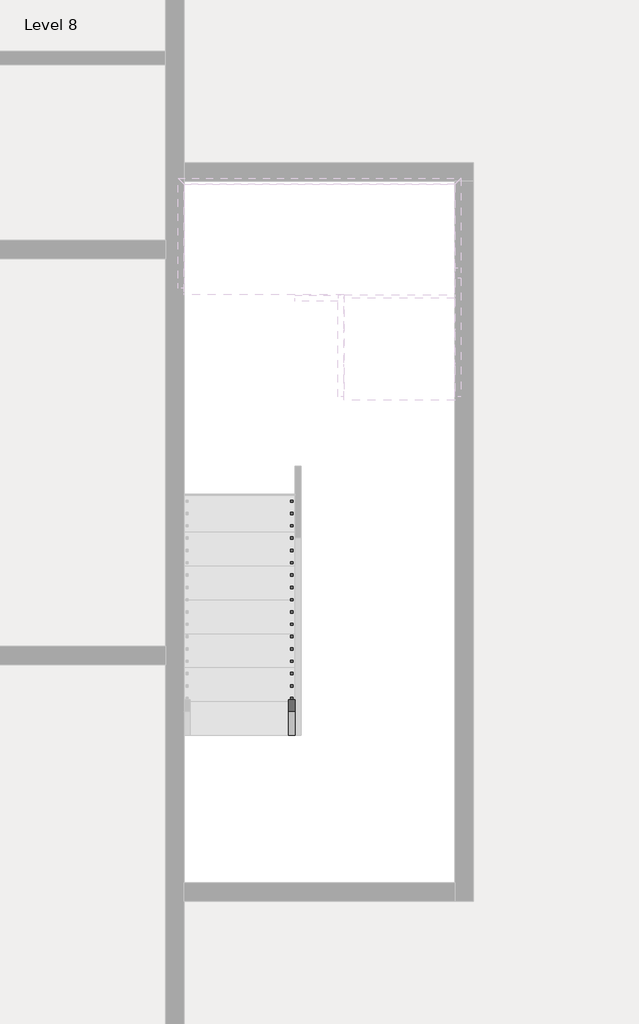
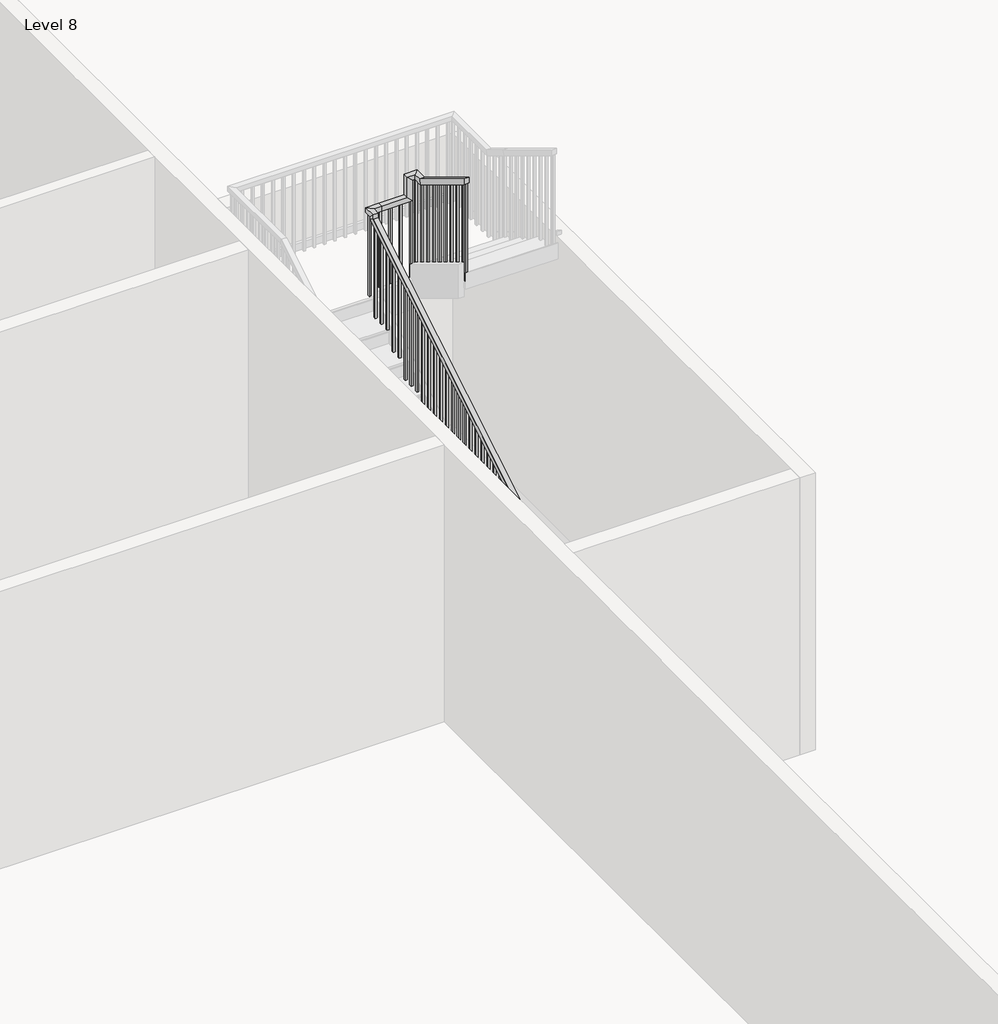
# One storey, part 5 of 8: 1 railing.
"""IFC4 building model written with IfcOpenShell, lengths in millimetres."""

from ifc_helpers import new_model, si_unit, frame, origin, place, context, project, spatial, polyline, outline, extrude, faceted_brep, element, save

model = new_model("IFC4")

# Units and contexts
model_context = context("Model", 3, world=origin())
ifc_project = project(units=[si_unit("LENGTHUNIT", "METRE", prefix="MILLI")], contexts=[model_context])

# Site, building, storey
site = spatial("IfcSite", under=ifc_project)
building = spatial("IfcBuilding", under=site)
storey = spatial("IfcBuildingStorey", under=building, Name="Level 8", Elevation=46570.6172466)

# Railing
placement = place(None, origin())
element("IfcRailing", 1, ObjectType="Handrail - Rectangular", at=placement, inside=storey, context=model_context, shape_type="SolidModel", body=[
    faceted_brep([(-2753.8415084, -23154.3851539, 47654.3505799), (-2753.8415084, -23154.3851539, 47594.9491197), (-2703.0415084, -23154.3851539, 47594.9491197), (-2703.0415084, -23154.3851539, 47654.3505799), (-2753.8415084, -19598.3851539, 49809.5020951), (-2753.8415084, -19547.5851539, 49780.8885136), (-2703.0415084, -19547.5851539, 49780.8885136), (-2703.0415084, -19598.3851539, 49809.5020951), (-2753.8415084, -19598.3851539, 49855.6839133), (-2753.8415084, -19547.5851539, 49804.8839133), (-2703.0415084, -19547.5851539, 49804.8839133), (-2703.0415084, -19598.3851539, 49855.6839133), (-2753.8415084, -19471.3851539, 49855.6839133), (-2753.8415084, -19471.3851539, 49804.8839133), (-2703.0415084, -19522.1851539, 49804.8839133), (-2703.0415084, -19522.1851539, 49855.6839133), (-2626.8415084, -19471.3851539, 49855.6839133), (-2626.8415084, -19471.3851539, 49804.8839133), (-2626.8415084, -19522.1851539, 49804.8839133), (-2626.8415084, -19522.1851539, 49855.6839133), (-2372.8415084, -19471.3851539, 49855.6839133), (-2322.0415084, -19471.3851539, 49804.8839133), (-2322.0415084, -19522.1851539, 49804.8839133), (-2372.8415084, -19522.1851539, 49855.6839133), (-2372.8415084, -19471.3851539, 50071.1990648), (-2322.0415084, -19471.3851539, 50020.3990648), (-2322.0415084, -19522.1851539, 50020.3990648), (-2372.8415084, -19522.1851539, 50071.1990648), (-2245.8415084, -19471.3851539, 50071.1990648), (-2245.8415084, -19471.3851539, 50020.3990648), (-2296.6415084, -19522.1851539, 50020.3990648), (-2296.6415084, -19522.1851539, 50071.1990648), (-2245.8415084, -19598.3851539, 50071.1990648), (-2245.8415084, -19612.5775633, 50020.3990648), (-2296.6415084, -19612.5775633, 50020.3990648), (-2296.6415084, -19598.3851539, 50071.1990648), (-2245.8415084, -20360.3851539, 50533.0172466), (-2296.6415084, -20360.3851539, 50533.0172466), (-2296.6415084, -20360.3851539, 50473.6157863), (-2245.8415084, -20360.3851539, 50473.6157863)], [[[0, 1, 2, 3]], [[1, 0, 4, 5]], [[2, 1, 5, 6]], [[3, 2, 6, 7]], [[0, 3, 7, 4]], [[5, 4, 8, 9]], [[6, 5, 9, 10]], [[7, 6, 10, 11]], [[4, 7, 11, 8]], [[9, 8, 12, 13]], [[10, 9, 13, 14]], [[11, 10, 14, 15]], [[8, 11, 15, 12]], [[13, 12, 16, 17]], [[14, 13, 17, 18]], [[15, 14, 18, 19]], [[12, 15, 19, 16]], [[17, 16, 20, 21]], [[18, 17, 21, 22]], [[19, 18, 22, 23]], [[16, 19, 23, 20]], [[21, 20, 24, 25]], [[22, 21, 25, 26]], [[23, 22, 26, 27]], [[20, 23, 27, 24]], [[25, 24, 28, 29]], [[26, 25, 29, 30]], [[27, 26, 30, 31]], [[24, 27, 31, 28]], [[29, 28, 32, 33]], [[30, 29, 33, 34]], [[31, 30, 34, 35]], [[28, 31, 35, 32]], [[36, 37, 38, 39]], [[33, 32, 36, 39]], [[34, 33, 39, 38]], [[35, 34, 38, 37]], [[32, 35, 37, 36]]]),
    extrude(outline(polyline([(-20319.1101539, 50448.6006348), (-20300.0601539, 50437.0551803), (-20300.0601539, 49449.2839133), (-20319.1101539, 49449.2839133), (-20319.1101539, 50448.6006348)])), frame((-2280.7665084, 0.0, 0.0), z_axis=(1.0, 0.0, 0.0), x_axis=(0.0, 1.0, 0.0)), (0.0, 0.0, 1.0), 19.05),
    extrude(outline(polyline([(-20217.5101539, 50387.0248773), (-20198.4601539, 50375.4794227), (-20198.4601539, 49449.2839133), (-20217.5101539, 49449.2839133), (-20217.5101539, 50387.0248773)])), frame((-2280.7665084, 0.0, 0.0), z_axis=(1.0, 0.0, 0.0), x_axis=(0.0, 1.0, 0.0)), (0.0, 0.0, 1.0), 19.05),
    extrude(outline(polyline([(-20115.9101539, 50325.4491197), (-20096.8601539, 50313.9036651), (-20096.8601539, 49449.2839133), (-20115.9101539, 49449.2839133), (-20115.9101539, 50325.4491197)])), frame((-2280.7665084, 0.0, 0.0), z_axis=(1.0, 0.0, 0.0), x_axis=(0.0, 1.0, 0.0)), (0.0, 0.0, 1.0), 19.05),
    extrude(outline(polyline([(-20014.3101539, 50263.8733621), (-19995.2601539, 50252.3279076), (-19995.2601539, 49279.9505799), (-20014.3101539, 49279.9505799), (-20014.3101539, 50263.8733621)])), frame((-2280.7665084, 0.0, 0.0), z_axis=(1.0, 0.0, 0.0), x_axis=(0.0, 1.0, 0.0)), (0.0, 0.0, 1.0), 19.05),
    extrude(outline(polyline([(-19912.7101539, 50202.2976045), (-19893.6601539, 50190.75215), (-19893.6601539, 49279.9505799), (-19912.7101539, 49279.9505799), (-19912.7101539, 50202.2976045)])), frame((-2280.7665084, 0.0, 0.0), z_axis=(1.0, 0.0, 0.0), x_axis=(0.0, 1.0, 0.0)), (0.0, 0.0, 1.0), 19.05),
    extrude(outline(polyline([(-19811.1101539, 50140.721847), (-19792.0601539, 50129.1763924), (-19792.0601539, 49279.9505799), (-19811.1101539, 49279.9505799), (-19811.1101539, 50140.721847)])), frame((-2280.7665084, 0.0, 0.0), z_axis=(1.0, 0.0, 0.0), x_axis=(0.0, 1.0, 0.0)), (0.0, 0.0, 1.0), 19.05),
    extrude(outline(polyline([(-19709.5101539, 50079.1460894), (-19690.4601539, 50067.6006348), (-19690.4601539, 49110.6172466), (-19709.5101539, 49110.6172466), (-19709.5101539, 50079.1460894)])), frame((-2280.7665084, 0.0, 0.0), z_axis=(1.0, 0.0, 0.0), x_axis=(0.0, 1.0, 0.0)), (0.0, 0.0, 1.0), 19.05),
    extrude(outline(polyline([(-19607.9101539, 50017.5703318), (-19588.8601539, 50006.0248773), (-19588.8601539, 49110.6172466), (-19607.9101539, 49110.6172466), (-19607.9101539, 50017.5703318)])), frame((-2280.7665084, 0.0, 0.0), z_axis=(1.0, 0.0, 0.0), x_axis=(0.0, 1.0, 0.0)), (0.0, 0.0, 1.0), 19.05),
    extrude(outline(polyline([(-2331.5665084, -19506.3101539), (-2331.5665084, -19487.2601539), (-2312.5165084, -19487.2601539), (-2312.5165084, -19506.3101539), (-2331.5665084, -19506.3101539)])), frame((0.0, 0.0, 48941.2839133), z_axis=(0.0, 0.0, 1.0), x_axis=(1.0, 0.0, 0.0)), (0.0, 0.0, 1.0), 1079.1151515),
    extrude(outline(polyline([(-2433.1665084, -19506.3101539), (-2433.1665084, -19487.2601539), (-2414.1165084, -19487.2601539), (-2414.1165084, -19506.3101539), (-2433.1665084, -19506.3101539)])), frame((0.0, 0.0, 48941.2839133), z_axis=(0.0, 0.0, 1.0), x_axis=(1.0, 0.0, 0.0)), (0.0, 0.0, 1.0), 863.6),
    extrude(outline(polyline([(-2534.7665084, -19506.3101539), (-2534.7665084, -19487.2601539), (-2515.7165084, -19487.2601539), (-2515.7165084, -19506.3101539), (-2534.7665084, -19506.3101539)])), frame((0.0, 0.0, 48941.2839133), z_axis=(0.0, 0.0, 1.0), x_axis=(1.0, 0.0, 0.0)), (0.0, 0.0, 1.0), 863.6),
    extrude(outline(polyline([(-2636.3665084, -19506.3101539), (-2636.3665084, -19487.2601539), (-2617.3165084, -19487.2601539), (-2617.3165084, -19506.3101539), (-2636.3665084, -19506.3101539)])), frame((0.0, 0.0, 48941.2839133), z_axis=(0.0, 0.0, 1.0), x_axis=(1.0, 0.0, 0.0)), (0.0, 0.0, 1.0), 863.6),
    extrude(outline(polyline([(-19607.9101539, 49744.3279076), (-19588.8601539, 49755.8733621), (-19588.8601539, 48771.9505799), (-19607.9101539, 48771.9505799), (-19607.9101539, 49744.3279076)])), frame((-2737.9665084, 0.0, 0.0), z_axis=(1.0, 0.0, 0.0), x_axis=(0.0, 1.0, 0.0)), (0.0, 0.0, 1.0), 19.05),
    extrude(outline(polyline([(-19709.5101539, 49682.75215), (-19690.4601539, 49694.2976045), (-19690.4601539, 48771.9505799), (-19709.5101539, 48771.9505799), (-19709.5101539, 49682.75215)])), frame((-2737.9665084, 0.0, 0.0), z_axis=(1.0, 0.0, 0.0), x_axis=(0.0, 1.0, 0.0)), (0.0, 0.0, 1.0), 19.05),
    extrude(outline(polyline([(-19811.1101539, 49621.1763924), (-19792.0601539, 49632.721847), (-19792.0601539, 48771.9505799), (-19811.1101539, 48771.9505799), (-19811.1101539, 49621.1763924)])), frame((-2737.9665084, 0.0, 0.0), z_axis=(1.0, 0.0, 0.0), x_axis=(0.0, 1.0, 0.0)), (0.0, 0.0, 1.0), 19.05),
    extrude(outline(polyline([(-19912.7101539, 49559.6006348), (-19893.6601539, 49571.1460894), (-19893.6601539, 48602.6172466), (-19912.7101539, 48602.6172466), (-19912.7101539, 49559.6006348)])), frame((-2737.9665084, 0.0, 0.0), z_axis=(1.0, 0.0, 0.0), x_axis=(0.0, 1.0, 0.0)), (0.0, 0.0, 1.0), 19.05),
    extrude(outline(polyline([(-20014.3101539, 49498.0248773), (-19995.2601539, 49509.5703318), (-19995.2601539, 48602.6172466), (-20014.3101539, 48602.6172466), (-20014.3101539, 49498.0248773)])), frame((-2737.9665084, 0.0, 0.0), z_axis=(1.0, 0.0, 0.0), x_axis=(0.0, 1.0, 0.0)), (0.0, 0.0, 1.0), 19.05),
    extrude(outline(polyline([(-20115.9101539, 49436.4491197), (-20096.8601539, 49447.9945742), (-20096.8601539, 48433.2839133), (-20115.9101539, 48433.2839133), (-20115.9101539, 49436.4491197)])), frame((-2737.9665084, 0.0, 0.0), z_axis=(1.0, 0.0, 0.0), x_axis=(0.0, 1.0, 0.0)), (0.0, 0.0, 1.0), 19.05),
    extrude(outline(polyline([(-20217.5101539, 49374.8733621), (-20198.4601539, 49386.4188166), (-20198.4601539, 48433.2839133), (-20217.5101539, 48433.2839133), (-20217.5101539, 49374.8733621)])), frame((-2737.9665084, 0.0, 0.0), z_axis=(1.0, 0.0, 0.0), x_axis=(0.0, 1.0, 0.0)), (0.0, 0.0, 1.0), 19.05),
    extrude(outline(polyline([(-20319.1101539, 49313.2976045), (-20300.0601539, 49324.8430591), (-20300.0601539, 48433.2839133), (-20319.1101539, 48433.2839133), (-20319.1101539, 49313.2976045)])), frame((-2737.9665084, 0.0, 0.0), z_axis=(1.0, 0.0, 0.0), x_axis=(0.0, 1.0, 0.0)), (0.0, 0.0, 1.0), 19.05),
    extrude(outline(polyline([(-20420.7101539, 49251.721847), (-20401.6601539, 49263.2673015), (-20401.6601539, 48263.9505799), (-20420.7101539, 48263.9505799), (-20420.7101539, 49251.721847)])), frame((-2737.9665084, 0.0, 0.0), z_axis=(1.0, 0.0, 0.0), x_axis=(0.0, 1.0, 0.0)), (0.0, 0.0, 1.0), 19.05),
    extrude(outline(polyline([(-20522.3101539, 49190.1460894), (-20503.2601539, 49201.6915439), (-20503.2601539, 48263.9505799), (-20522.3101539, 48263.9505799), (-20522.3101539, 49190.1460894)])), frame((-2737.9665084, 0.0, 0.0), z_axis=(1.0, 0.0, 0.0), x_axis=(0.0, 1.0, 0.0)), (0.0, 0.0, 1.0), 19.05),
    extrude(outline(polyline([(-20623.9101539, 49128.5703318), (-20604.8601539, 49140.1157863), (-20604.8601539, 48263.9505799), (-20623.9101539, 48263.9505799), (-20623.9101539, 49128.5703318)])), frame((-2737.9665084, 0.0, 0.0), z_axis=(1.0, 0.0, 0.0), x_axis=(0.0, 1.0, 0.0)), (0.0, 0.0, 1.0), 19.05),
    extrude(outline(polyline([(-20725.5101539, 49066.9945742), (-20706.4601539, 49078.5400288), (-20706.4601539, 48094.6172466), (-20725.5101539, 48094.6172466), (-20725.5101539, 49066.9945742)])), frame((-2737.9665084, 0.0, 0.0), z_axis=(1.0, 0.0, 0.0), x_axis=(0.0, 1.0, 0.0)), (0.0, 0.0, 1.0), 19.05),
    extrude(outline(polyline([(-20827.1101539, 49005.4188166), (-20808.0601539, 49016.9642712), (-20808.0601539, 48094.6172466), (-20827.1101539, 48094.6172466), (-20827.1101539, 49005.4188166)])), frame((-2737.9665084, 0.0, 0.0), z_axis=(1.0, 0.0, 0.0), x_axis=(0.0, 1.0, 0.0)), (0.0, 0.0, 1.0), 19.05),
    extrude(outline(polyline([(-20928.7101539, 48943.8430591), (-20909.6601539, 48955.3885136), (-20909.6601539, 48094.6172466), (-20928.7101539, 48094.6172466), (-20928.7101539, 48943.8430591)])), frame((-2737.9665084, 0.0, 0.0), z_axis=(1.0, 0.0, 0.0), x_axis=(0.0, 1.0, 0.0)), (0.0, 0.0, 1.0), 19.05),
    extrude(outline(polyline([(-21030.3101539, 48882.2673015), (-21011.2601539, 48893.812756), (-21011.2601539, 47925.2839133), (-21030.3101539, 47925.2839133), (-21030.3101539, 48882.2673015)])), frame((-2737.9665084, 0.0, 0.0), z_axis=(1.0, 0.0, 0.0), x_axis=(0.0, 1.0, 0.0)), (0.0, 0.0, 1.0), 19.05),
    extrude(outline(polyline([(-21131.9101539, 48820.6915439), (-21112.8601539, 48832.2369985), (-21112.8601539, 47925.2839133), (-21131.9101539, 47925.2839133), (-21131.9101539, 48820.6915439)])), frame((-2737.9665084, 0.0, 0.0), z_axis=(1.0, 0.0, 0.0), x_axis=(0.0, 1.0, 0.0)), (0.0, 0.0, 1.0), 19.05),
    extrude(outline(polyline([(-21233.5101539, 48759.1157863), (-21214.4601539, 48770.6612409), (-21214.4601539, 47755.9505799), (-21233.5101539, 47755.9505799), (-21233.5101539, 48759.1157863)])), frame((-2737.9665084, 0.0, 0.0), z_axis=(1.0, 0.0, 0.0), x_axis=(0.0, 1.0, 0.0)), (0.0, 0.0, 1.0), 19.05),
    extrude(outline(polyline([(-21335.1101539, 48697.5400288), (-21316.0601539, 48709.0854833), (-21316.0601539, 47755.9505799), (-21335.1101539, 47755.9505799), (-21335.1101539, 48697.5400288)])), frame((-2737.9665084, 0.0, 0.0), z_axis=(1.0, 0.0, 0.0), x_axis=(0.0, 1.0, 0.0)), (0.0, 0.0, 1.0), 19.05),
    extrude(outline(polyline([(-21436.7101539, 48635.9642712), (-21417.6601539, 48647.5097257), (-21417.6601539, 47755.9505799), (-21436.7101539, 47755.9505799), (-21436.7101539, 48635.9642712)])), frame((-2737.9665084, 0.0, 0.0), z_axis=(1.0, 0.0, 0.0), x_axis=(0.0, 1.0, 0.0)), (0.0, 0.0, 1.0), 19.05),
    extrude(outline(polyline([(-21538.3101539, 48574.3885136), (-21519.2601539, 48585.9339682), (-21519.2601539, 47586.6172466), (-21538.3101539, 47586.6172466), (-21538.3101539, 48574.3885136)])), frame((-2737.9665084, 0.0, 0.0), z_axis=(1.0, 0.0, 0.0), x_axis=(0.0, 1.0, 0.0)), (0.0, 0.0, 1.0), 19.05),
    extrude(outline(polyline([(-21639.9101539, 48512.812756), (-21620.8601539, 48524.3582106), (-21620.8601539, 47586.6172466), (-21639.9101539, 47586.6172466), (-21639.9101539, 48512.812756)])), frame((-2737.9665084, 0.0, 0.0), z_axis=(1.0, 0.0, 0.0), x_axis=(0.0, 1.0, 0.0)), (0.0, 0.0, 1.0), 19.05),
    extrude(outline(polyline([(-21741.5101539, 48451.2369985), (-21722.4601539, 48462.782453), (-21722.4601539, 47586.6172466), (-21741.5101539, 47586.6172466), (-21741.5101539, 48451.2369985)])), frame((-2737.9665084, 0.0, 0.0), z_axis=(1.0, 0.0, 0.0), x_axis=(0.0, 1.0, 0.0)), (0.0, 0.0, 1.0), 19.05),
    extrude(outline(polyline([(-21843.1101539, 48389.6612409), (-21824.0601539, 48401.2066954), (-21824.0601539, 47417.2839133), (-21843.1101539, 47417.2839133), (-21843.1101539, 48389.6612409)])), frame((-2737.9665084, 0.0, 0.0), z_axis=(1.0, 0.0, 0.0), x_axis=(0.0, 1.0, 0.0)), (0.0, 0.0, 1.0), 19.05),
    extrude(outline(polyline([(-21944.7101539, 48328.0854833), (-21925.6601539, 48339.6309379), (-21925.6601539, 47417.2839133), (-21944.7101539, 47417.2839133), (-21944.7101539, 48328.0854833)])), frame((-2737.9665084, 0.0, 0.0), z_axis=(1.0, 0.0, 0.0), x_axis=(0.0, 1.0, 0.0)), (0.0, 0.0, 1.0), 19.05),
    extrude(outline(polyline([(-22046.3101539, 48266.5097257), (-22027.2601539, 48278.0551803), (-22027.2601539, 47417.2839133), (-22046.3101539, 47417.2839133), (-22046.3101539, 48266.5097257)])), frame((-2737.9665084, 0.0, 0.0), z_axis=(1.0, 0.0, 0.0), x_axis=(0.0, 1.0, 0.0)), (0.0, 0.0, 1.0), 19.05),
    extrude(outline(polyline([(-22147.9101539, 48204.9339682), (-22128.8601539, 48216.4794227), (-22128.8601539, 47247.9505799), (-22147.9101539, 47247.9505799), (-22147.9101539, 48204.9339682)])), frame((-2737.9665084, 0.0, 0.0), z_axis=(1.0, 0.0, 0.0), x_axis=(0.0, 1.0, 0.0)), (0.0, 0.0, 1.0), 19.05),
    extrude(outline(polyline([(-22249.5101539, 48143.3582106), (-22230.4601539, 48154.9036651), (-22230.4601539, 47247.9505799), (-22249.5101539, 47247.9505799), (-22249.5101539, 48143.3582106)])), frame((-2737.9665084, 0.0, 0.0), z_axis=(1.0, 0.0, 0.0), x_axis=(0.0, 1.0, 0.0)), (0.0, 0.0, 1.0), 19.05),
    extrude(outline(polyline([(-22351.1101539, 48081.782453), (-22332.0601539, 48093.3279076), (-22332.0601539, 47078.6172466), (-22351.1101539, 47078.6172466), (-22351.1101539, 48081.782453)])), frame((-2737.9665084, 0.0, 0.0), z_axis=(1.0, 0.0, 0.0), x_axis=(0.0, 1.0, 0.0)), (0.0, 0.0, 1.0), 19.05),
    extrude(outline(polyline([(-22452.7101539, 48020.2066954), (-22433.6601539, 48031.75215), (-22433.6601539, 47078.6172466), (-22452.7101539, 47078.6172466), (-22452.7101539, 48020.2066954)])), frame((-2737.9665084, 0.0, 0.0), z_axis=(1.0, 0.0, 0.0), x_axis=(0.0, 1.0, 0.0)), (0.0, 0.0, 1.0), 19.05),
    extrude(outline(polyline([(-22554.3101539, 47958.6309379), (-22535.2601539, 47970.1763924), (-22535.2601539, 47078.6172466), (-22554.3101539, 47078.6172466), (-22554.3101539, 47958.6309379)])), frame((-2737.9665084, 0.0, 0.0), z_axis=(1.0, 0.0, 0.0), x_axis=(0.0, 1.0, 0.0)), (0.0, 0.0, 1.0), 19.05),
    extrude(outline(polyline([(-22655.9101539, 47897.0551803), (-22636.8601539, 47908.6006348), (-22636.8601539, 46909.2839133), (-22655.9101539, 46909.2839133), (-22655.9101539, 47897.0551803)])), frame((-2737.9665084, 0.0, 0.0), z_axis=(1.0, 0.0, 0.0), x_axis=(0.0, 1.0, 0.0)), (0.0, 0.0, 1.0), 19.05),
    extrude(outline(polyline([(-22757.5101539, 47835.4794227), (-22738.4601539, 47847.0248773), (-22738.4601539, 46909.2839133), (-22757.5101539, 46909.2839133), (-22757.5101539, 47835.4794227)])), frame((-2737.9665084, 0.0, 0.0), z_axis=(1.0, 0.0, 0.0), x_axis=(0.0, 1.0, 0.0)), (0.0, 0.0, 1.0), 19.05),
    extrude(outline(polyline([(-22859.1101539, 47773.9036651), (-22840.0601539, 47785.4491197), (-22840.0601539, 46909.2839133), (-22859.1101539, 46909.2839133), (-22859.1101539, 47773.9036651)])), frame((-2737.9665084, 0.0, 0.0), z_axis=(1.0, 0.0, 0.0), x_axis=(0.0, 1.0, 0.0)), (0.0, 0.0, 1.0), 19.05),
    extrude(outline(polyline([(-22960.7101539, 47712.3279076), (-22941.6601539, 47723.8733621), (-22941.6601539, 46739.9505799), (-22960.7101539, 46739.9505799), (-22960.7101539, 47712.3279076)])), frame((-2737.9665084, 0.0, 0.0), z_axis=(1.0, 0.0, 0.0), x_axis=(0.0, 1.0, 0.0)), (0.0, 0.0, 1.0), 19.05),
    extrude(outline(polyline([(-23062.3101539, 47650.75215), (-23043.2601539, 47662.2976045), (-23043.2601539, 46739.9505799), (-23062.3101539, 46739.9505799), (-23062.3101539, 47650.75215)])), frame((-2737.9665084, 0.0, 0.0), z_axis=(1.0, 0.0, 0.0), x_axis=(0.0, 1.0, 0.0)), (0.0, 0.0, 1.0), 19.05),
    extrude(outline(polyline([(-2280.7665084, -19506.3101539), (-2280.7665084, -19487.2601539), (-2261.7165084, -19487.2601539), (-2261.7165084, -19506.3101539), (-2280.7665084, -19506.3101539)])), frame((0.0, 0.0, 48941.2839133), z_axis=(0.0, 0.0, 1.0), x_axis=(1.0, 0.0, 0.0)), (0.0, 0.0, 1.0), 1079.1151515),
    extrude(outline(polyline([(-2718.9165084, -19506.3101539), (-2737.9665084, -19506.3101539), (-2737.9665084, -19487.2601539), (-2718.9165084, -19487.2601539), (-2718.9165084, -19506.3101539)])), frame((0.0, 0.0, 48941.2839133), z_axis=(0.0, 0.0, 1.0), x_axis=(1.0, 0.0, 0.0)), (0.0, 0.0, 1.0), 863.6),
    extrude(outline(polyline([(-20360.3851539, 50473.6157863), (-20341.3351539, 50462.0703318), (-20341.3351539, 49449.2839133), (-20360.3851539, 49449.2839133), (-20360.3851539, 50473.6157863)])), frame((-2280.7665084, 0.0, 0.0), z_axis=(1.0, 0.0, 0.0), x_axis=(0.0, 1.0, 0.0)), (0.0, 0.0, 1.0), 19.05),
    extrude(outline(polyline([(-23154.3851539, 47594.9491197), (-23135.3351539, 47606.4945742), (-23135.3351539, 46739.9505799), (-23154.3851539, 46739.9505799), (-23154.3851539, 47594.9491197)])), frame((-2737.9665084, 0.0, 0.0), z_axis=(1.0, 0.0, 0.0), x_axis=(0.0, 1.0, 0.0)), (0.0, 0.0, 1.0), 19.05),
])

save(model, "model.ifc")

# Revit data of these elements
# Type "Handrail - Rectangular"
#   Assembly Code = "C2010400"
#   built-in parameter 1008612 = 0.0416667 (stored number, unit not read)
#   built-in parameter 1008611 = 0.0416667 (stored number, unit not read)
#   built-in parameter 1008609 = 0.333333 (stored number, unit not read)
#   built-in parameter 1008604 = 0.166667 (stored number, unit not read)
#   built-in parameter 1008603 = 0.166667 (stored number, unit not read)
#   Railing Height = 3' - 0"
#   built-in parameter 1008630 = 2
#   built-in parameter 1008610 = 2
#   built-in parameter 1008618 = Baluster - Square : 3/4"
# Element 1 (IfcRailing, "Handrail - Rectangular")
#   Phase Created = New Construction
